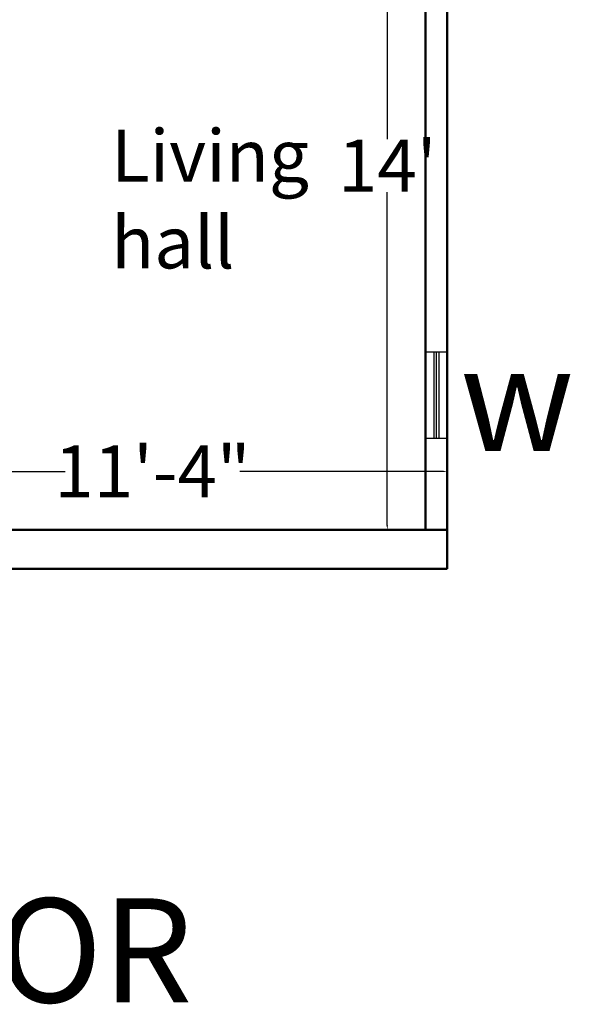
# Model space of a CAD drawing. Units: inches. Extents: x 409 to 7572, y 7 to 725.
# Tile 18 of 38: x 3250 to 3378, y 56 to 283. Entities that reach past the tile are written whole.
import ezdxf

# ---------------------------------------------------------------- set-up
doc = ezdxf.new("R2010")
doc.units = ezdxf.units.IN
doc.header["$MEASUREMENT"] = 0
for name, color, linetype, lineweight in [('A-ANNO-DIMS', 2, 'Continuous', 18), ('A-ANNO-SYMB', 3, 'Continuous', 25), ('A-ANNO-TEXT', 7, 'Continuous', 35), ('A-AREA-IDEN', 7, 'Continuous', 25), ('A-GLAZ', 4, 'Continuous', 25), ('A-WALL', 7, 'Continuous', 50)]:
    doc.layers.add(name, color=color, linetype=linetype, lineweight=lineweight)
doc.styles.get("Standard").update_dxf_attribs({"font": 'arial.ttf'})
doc.dimstyles.get("Standard").update_dxf_attribs({"dimtxt": 2, "dimasz": 1, "dimexe": 0.18, "dimexo": 0.0625, "dimgap": 0.09, "dimtad": 0, "dimtih": 1, "dimtoh": 1, "dimdec": 0, "dimzin": 0, "dimdsep": 46, "dimlunit": 3, "dimtxsty": 'Standard', "dimcen": 0.09, "dimadec": 0, "dimazin": 0, "dimtfac": 1, "dimtdec": 0, "dimtofl": 0, "dimtmove": 0, "dimatfit": 3, "dimfxl": 1, "dimtolj": 1, "dimtzin": 0, "dimarcsym": 0})

# ---------------------------------------------------------------- blocks, each defined once
blk = doc.blocks.new('*D67')
at = {"layer": 'A-ANNO-DIMS', "color": 0, "lineweight": -2, "transparency": 16777216}
for p, q in [((3344.04, 333.53), (3335.1, 333.53)), ((3335.28, 332.53), (3335.28, 255.65)), ((3335.28, 166.53), (3335.28, 243.42)), ((3344.04, 165.53), (3335.1, 165.53))]:
    blk.add_line(p, q, dxfattribs=at)
at = {"layer": 'A-ANNO-DIMS', "color": 0, "transparency": 16777216}
for points in [[(3335.12, 332.53), (3335.45, 332.53), (3335.28, 333.53)], [(3335.12, 166.53), (3335.45, 166.53), (3335.28, 165.53)]]:
    blk.add_solid(points, dxfattribs=at)
at = {"layer": 'DEFPOINTS', "color": 0, "transparency": 16777216}
for p in [(3344.1, 333.53), (3335.28, 165.53), (3344.1, 165.53)]:
    blk.add_point(p, dxfattribs=at)
at = {"layer": 'A-ANNO-DIMS', "color": 0, "transparency": 16777216, "insert": (3335.28, 249.53), "char_height": 2, "attachment_point": 5}
blk.add_mtext("\\A1;{\\H6x;14'}", dxfattribs=at)
blk = doc.blocks.new('*D68')
at = {"layer": 'A-ANNO-DIMS', "color": 0, "lineweight": -2, "transparency": 16777216}
for p, q in [((3213.1, 165.59), (3213.1, 179.18)), ((3214.1, 179), (3260.96, 179)), ((3348.1, 179), (3301.23, 179)), ((3349.1, 165.59), (3349.1, 179.18))]:
    blk.add_line(p, q, dxfattribs=at)
at = {"layer": 'A-ANNO-DIMS', "color": 0, "transparency": 16777216}
for points in [[(3214.1, 179.16), (3214.1, 178.83), (3213.1, 179)], [(3348.1, 179.16), (3348.1, 178.83), (3349.1, 179)]]:
    blk.add_solid(points, dxfattribs=at)
at = {"layer": 'DEFPOINTS', "color": 0, "transparency": 16777216}
for p in [(3349.1, 179), (3213.1, 165.53), (3349.1, 165.53)]:
    blk.add_point(p, dxfattribs=at)
at = {"layer": 'A-ANNO-DIMS', "color": 0, "transparency": 16777216, "insert": (3281.1, 179), "char_height": 2, "attachment_point": 5}
blk.add_mtext('\\A1;{\\H6x;11\'-4"}', dxfattribs=at)
blk = doc.blocks.new('WIN-20')
for p, q in [((2103.48, 182.68), (2083.54, 182.68)), ((2103.48, 182.13), (2083.54, 182.13)), ((2103.48, 181.57), (2083.54, 181.57))]:
    blk.add_line(p, q)
blk.add_lwpolyline([(2103.48, 179.64), (2083.54, 179.64), (2083.54, 184.62), (2103.48, 184.62)], close=True)

msp = doc.modelspace()

# ---------------------------------------------------------------- linework, layer by layer
at = {"layer": 'A-WALL'}
for p, q in [((3344.1, 333.53), (3344.1, 165.53)), ((3344.1, 333.53), (3344.1, 165.53)), ((3349.1, 315.53), (3349.1, 165.53)), ((3213.1, 165.53), (3349.1, 165.53)), ((3349.1, 165.53), (3349.1, 156.53)), ((2975.1, 156.53), (3349.1, 156.53))]:
    msp.add_line(p, q, dxfattribs=at)

# ---------------------------------------------------------------- block references
at = {"layer": 'A-GLAZ', "rotation": 89.99999999999905}
msp.add_blockref('WIN-20', (3528.73, -1896.94), dxfattribs=at)

# ---------------------------------------------------------------- texts
at = {"layer": 'A-ANNO-SYMB', "insert": (3352.1, 207.68), "char_height": 24, "attachment_point": 1}
msp.add_mtext_dynamic_manual_height_columns('w', width=18.2582, gutter_width=1, heights=[0], dxfattribs=at)
at = {"layer": 'A-ANNO-TEXT', "insert": (3047.61, 80.54), "char_height": 24, "attachment_point": 1}
msp.add_mtext_dynamic_manual_height_columns('SECOND FLOOR', width=577.2242, gutter_width=1, heights=[0], dxfattribs=at)
at = {"layer": 'A-AREA-IDEN', "insert": (3271.57, 257.83), "char_height": 12, "attachment_point": 1}
msp.add_mtext_dynamic_manual_height_columns('Living hall', width=58.8843, gutter_width=1, heights=[0], dxfattribs=at)

# ---------------------------------------------------------------- dimensions: what is measured, and where the dimension line sits
at = {"layer": 'A-ANNO-DIMS'}
dim = msp.add_linear_dim(base=(3335.28, 165.53), p1=(3344.1, 333.53), p2=(3344.1, 165.53), angle=90, text='{\\H6x;<>}', dimstyle='Standard', override={"dimclrd": 0, "dimclre": 0, "dimclrt": 0}, dxfattribs=at)
dim.commit()
dim.dimension.update_dxf_attribs({"geometry": '*D67', "text_midpoint": (3335.28, 249.53)})
dim = msp.add_linear_dim(base=(3349.1, 179), p1=(3213.1, 165.53), p2=(3349.1, 165.53), text='{\\H6x;<>}', dimstyle='Standard', override={"dimclrd": 0, "dimclre": 0, "dimclrt": 0}, dxfattribs=at)
dim.commit()
dim.dimension.update_dxf_attribs({"geometry": '*D68', "text_midpoint": (3281.1, 179)})

doc.saveas('drawing.dxf')
